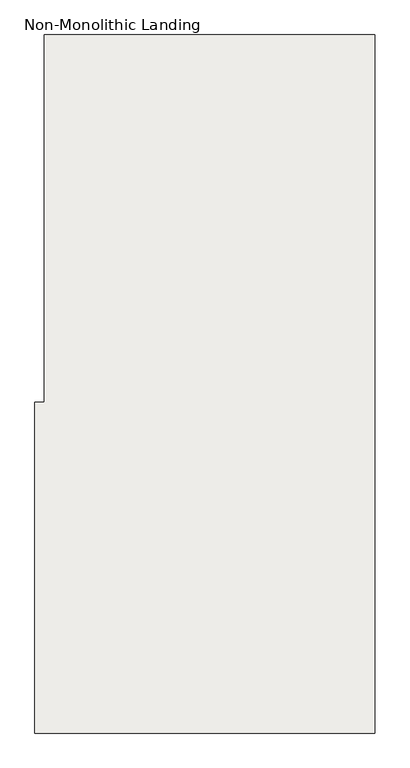
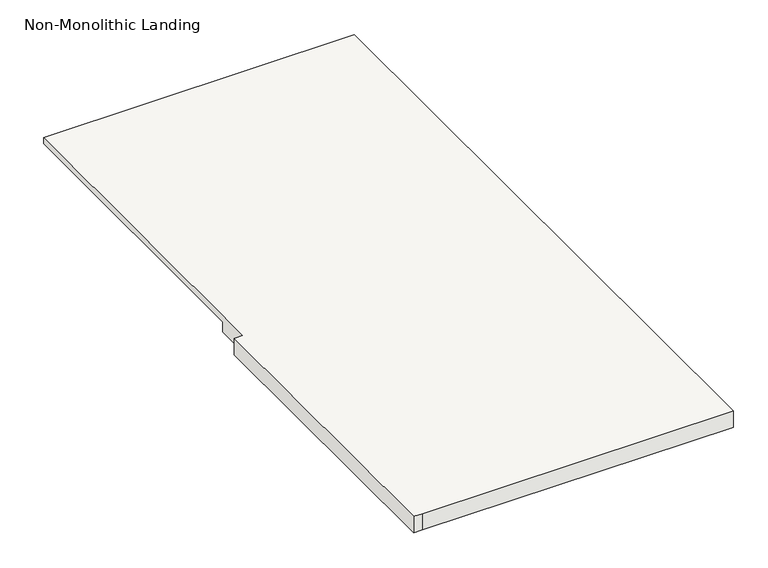
"""IFC4 building model written with IfcOpenShell, lengths in millimetres: slab geometry, Non-Monolithic Landing."""

from ifc_helpers import new_model, si_unit, origin, place, context, project, spatial, faceted_brep, source, transform, mapped, element, save


def non_monolithic_landing_f7b8efd9(model_context):
    return source(origin(), model_context, "Body", "Brep", [
        faceted_brep([(923.4845537, -3822.9544725, 7981.95), (948.8845537, -3822.9544725, 7956.55), (948.8845537, -4737.3544725, 7956.55), (923.4845537, -4737.3544725, 7981.95), (923.4845537, -4838.9544725, 8001.0), (898.0845537, -4838.9544725, 8001.0), (898.0845537, -5753.3544725, 8001.0), (923.4845537, -5753.3544725, 8001.0), (1837.8845537, -5753.3544725, 8001.0), (1837.8845537, -3822.9544725, 8001.0), (923.4845537, -3822.9544725, 8001.0), (948.8845537, -4737.3544725, 7950.2), (948.8845537, -3822.9544725, 7950.2), (1837.8845537, -3822.9544725, 7950.2), (1837.8845537, -5753.3544725, 7950.2), (923.4845537, -5753.3544725, 7950.2), (898.0845537, -5753.3544725, 7950.2), (898.0845537, -4838.9544725, 7950.2), (923.4845537, -4838.9544725, 7950.2), (923.4845537, -4737.3544725, 7950.2)], [[[0, 1, 2, 3]], [[4, 5, 6, 7, 8, 9, 10]], [[11, 12, 13, 14, 15, 16, 17, 18, 19]], [[12, 11, 2, 1]], [[11, 19, 3, 2]], [[4, 10, 0, 3, 19, 18]], [[5, 4, 18, 17]], [[6, 5, 17, 16]], [[7, 6, 16, 15]], [[8, 7, 15, 14]], [[9, 8, 14, 13]], [[10, 9, 13, 12, 1, 0]]]),
    ])


if __name__ == "__main__":
    model = new_model("IFC4")
    model_context = context("Model", 3, world=origin())
    ifc_project = project(units=[si_unit("LENGTHUNIT", "METRE", prefix="MILLI")], contexts=[model_context])
    site = spatial("IfcSite", under=ifc_project)
    building = spatial("IfcBuilding", under=site)
    placement = place(None, origin())
    non_monolithic_landing_shape = non_monolithic_landing_f7b8efd9(model_context)
    element("IfcSlab", 1, ObjectType="Non-Monolithic Landing", at=placement, inside=building, context=model_context, shape_type="MappedRepresentation", body=[
        mapped(non_monolithic_landing_shape, transform((0.0, 0.0, 0.0), x_axis=(1.0, 0.0, 0.0), y_axis=(0.0, 1.0, 0.0), z_axis=(0.0, 0.0, 1.0))),
    ])
    save(model, "model.ifc")
